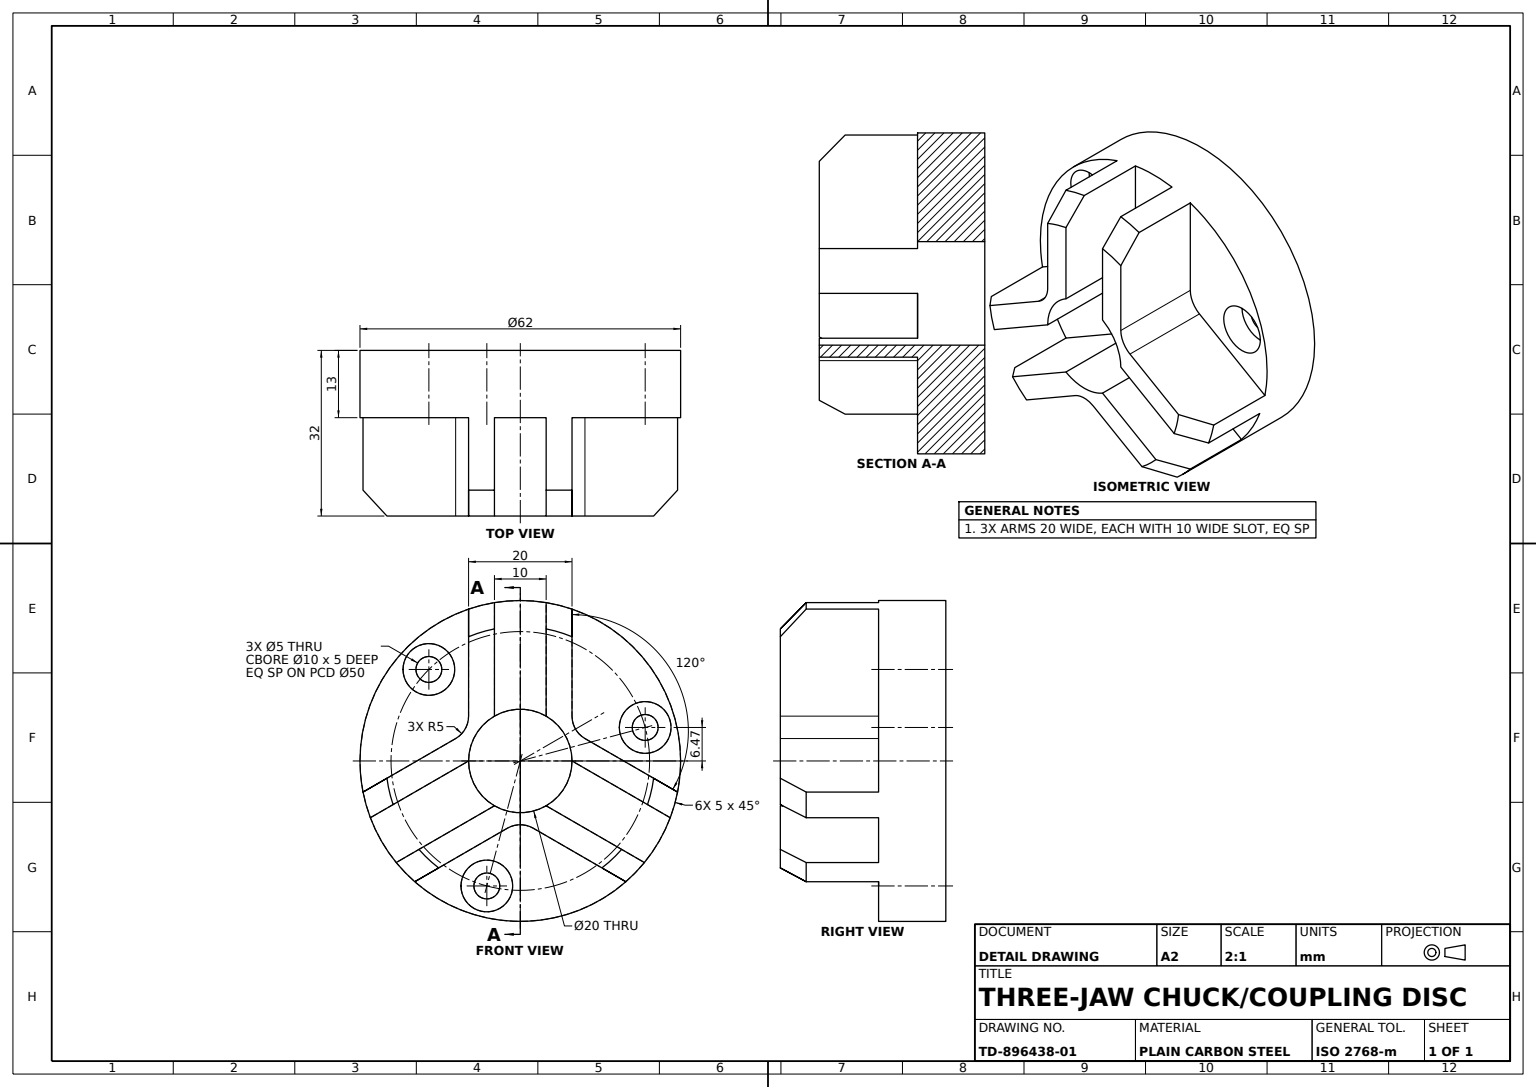
SolidWorks part; units mm, degrees
material "Plain Carbon Steel"
ref_plane "Front Plane" through (0, 0, 0) normal (0, 0, 1) x (1, 0, 0)
ref_plane "Top Plane" through (0, 0, 0) normal (0, 1, 0) x (1, 0, 0)
ref_plane "Right Plane" through (0, 0, 0) normal (1, 0, 0) x (0, 0, -1)
sketch "Base Disc Sketch" plane through (0, 0, 0) normal (0, 0, 1) x (1, 0, 0)
  circle A0 centre (0, 0) radius 31
  dimension "D1" = 62
extrude "Base Disc Ø62" add sketch "Base Disc Sketch" along normal blind 13
sketch "Relief Cut Sketch" plane through (0, 0, 13) normal (0, 0, 1) x (1, 0, 0)
  line L0 (0, 0) -> (0, 31) construction
  circle A0 centre (0, 0) radius 10
  circle A1 centre (0, 0) radius 31 construction
  dimension "D1" = 20
extrude "Relief Cut" cut sketch "Relief Cut Sketch" against normal through all
sketch "Arms Profile Sketch" plane through (0, 0, 13) normal (0, 0, 1) x (1, 0, 0)
  line L1 (10, 8.6603) -> (10, 29.3428)
  line L2 (-10, 8.6603) -> (-10, 29.3428)
  line L5 (-12.5, 4.3301) -> (-30.4116, -6.0111)
  line L8 (-2.5, -12.9904) -> (-20.4116, -23.3317)
  line L9 (0, 0) -> (10, 0) construction
  line L12 (2.5, -12.9904) -> (20.4116, -23.3317)
  line L13 (12.5, 4.3301) -> (30.4116, -6.0111)
  line L14 (0, 0) -> (-31, 0) construction
  line L18 (-10, 0) -> (-28.9953, -10.9669)
  line L19 (-5, -8.6603) -> (-23.9953, -19.6272)
  line L20 (5, -8.6603) -> (23.9953, -19.6272)
  line L23 (10, 0) -> (28.9953, -10.9669)
  line L24 (5, 8.6603) -> (5, 30.5941)
  line L27 (-5, 8.6603) -> (-5, 30.5941)
  circle A0 centre (0, 0) radius 31 construction
  arc A1 (-31, 0) -> (-20.4116, -23.3317) centre (0, 0) ccw
  arc A2 (-12.5, 4.3301) -> (-10, 8.6603) centre (-15, 8.6603) ccw
  arc A3 (10, 8.6603) -> (12.5, 4.3301) centre (15, 8.6603) ccw
  arc A4 (2.5, -12.9904) -> (-2.5, -12.9904) centre (0, -17.3205) ccw
  arc A5 (-10, 0) -> (-5, -8.6603) centre (0, 0) ccw
  arc A6 (5, 8.6603) -> (-5, 8.6603) centre (0, 0) ccw
  arc A7 (5, -8.6603) -> (10, 0) centre (0, 0) ccw
  arc A8 (20.4116, -23.3317) -> (30.4116, -6.0111) centre (0, 0) ccw
  arc A9 (10, 29.3428) -> (-10, 29.3428) centre (0, 0) ccw
  point P6 (10, 0)
  point P7 (10, 31)
  point P8 (-10, 0)
  point P9 (-10, 31)
  point P15 (-5, 8.6603)
  point P16 (-31.8468, -6.8397)
  point P17 (5, -8.6603)
  point P18 (-21.8468, -24.1603)
  point P23 (-5, -8.6603)
  point P26 (21.8468, -24.1603)
  point P27 (5, 8.6603)
  point P28 (31.8468, -6.8397)
  point P39 (-2.5, 4.3301)
  point P40 (-29.3468, -11.1699)
  point P41 (2.5, -4.3301)
  point P42 (-24.3468, -19.8301)
  point P45 (-2.5, -4.3301)
  point P47 (24.3468, -19.8301)
  point P48 (2.5, 4.3301)
  point P49 (29.3468, -11.1699)
  point P51 (5, 0)
  point P54 (-5, 0)
  circle M13 centre (0, 0) radius 10
  circle M14 centre (0, 0) radius 31
  dimension "D4" = 31
  dimension "D6" = 10
  dimension "D10" = 10
  dimension "D11" = 10
  dimension "D14" = 5
  dimension "D5" = 10
  dimension "D3" = 30.5941
  dimension "D7" = 20
  dimension "D12" = 20
  dimension "D2" = 30.5941
  dimension "D8" = 120
  dimension "D9" = 120
  dimension "D13" = 20
  dimension "D15" = 5
  dimension "D16" = 10
  dimension "D17" = 10
extrude "Three-Arm Boss" add sketch "Arms Profile Sketch" along normal blind 19 contours A2 L5 L18 L27 L2 M14 M13 | A3 L1 L24 L23 L13 M14 M13 | A4 L12 L20 L19 L8 M14 M13
sketch "Arm Gap Sketch" plane through (0, 0, 13) normal (0, 0, 1) x (1, 0, 0)
  line L0 (0, 0) -> (0, -31) construction
  line L1 (0, 0) -> (-8.0234, -29.9437) construction
  circle A0 centre (0, 0) radius 25 construction
  arc A1 (-20.4116, -23.3317) -> (20.4116, -23.3317) centre (0, 0) ccw construction
  circle A2 centre (-6.4705, -24.1481) radius 2.5
  dimension "D1" = 50
  dimension "D3" = 5
  dimension "D2" = 15
extrude "Arm Gap Cut" cut sketch "Arm Gap Sketch" against normal through all
sketch "Radial Hole Sketch" plane through (0, 0, 13) normal (0, 0, 1) x (1, 0, 0)
  circle A0 centre (-6.4705, -24.1481) radius 5
  dimension "D1" = 10
extrude "Radial Hole Ø10" cut sketch "Radial Hole Sketch" against normal blind 5
pattern_circular "Arm Cuts Pattern 3x" count 3 over 360 about axis through (0, 0, 0) along (0, 0, 1) of "Radial Hole Ø10", "Arm Gap Cut"
chamfer "Arm Chamfers 5mm" distance 5 angle 45 6 edges at (-22.2806, -21.554, 32) (22.2806, -21.554, 32) (29.8066, -8.5185, 32) (7.5261, 30.0726, 32) (-7.5261, 30.0726, 32) (-29.8066, -8.5185, 32)
